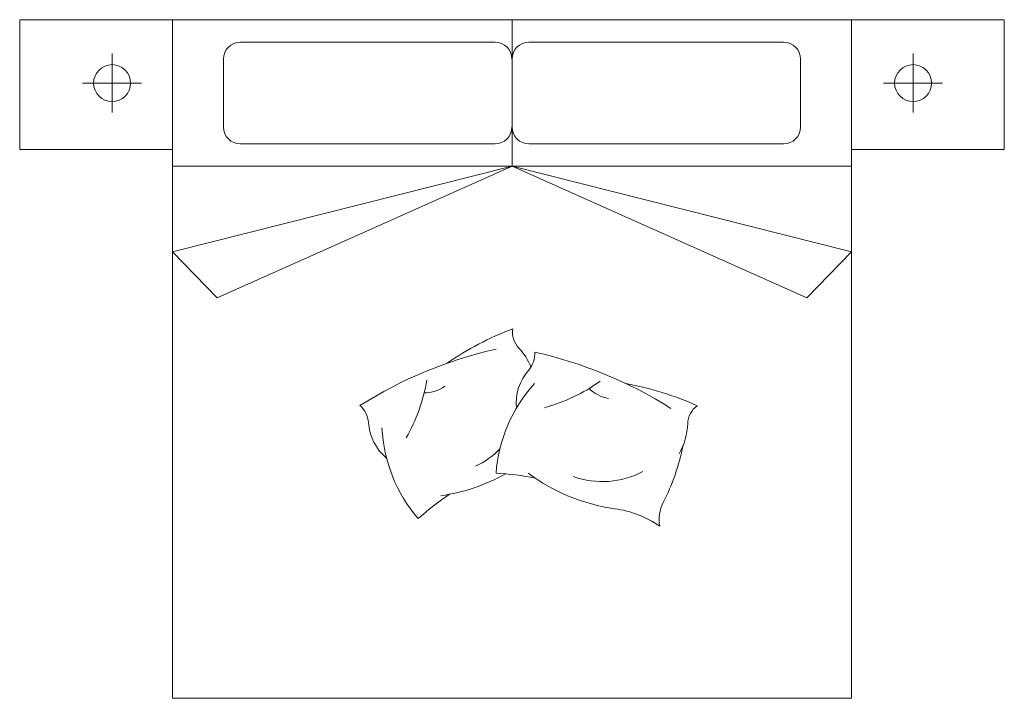
# Model space of a CAD drawing. Units: inches. Extents: x 1994 to 3075, y 3517 to 3950.
# Tile 9 of 58: x 1993.9962 to 1994.1, y 3553.8118 to 3553.8833. Entities that reach past the tile are written whole.
import ezdxf

# ---------------------------------------------------------------- set-up
doc = ezdxf.new("R2010")
doc.units = ezdxf.units.IN
doc.layers.add('A-FURN-REFR', color=8, linetype='Continuous', lineweight=13)

msp = doc.modelspace()

# ---------------------------------------------------------------- linework, layer by layer
at = {"layer": 'A-FURN-REFR'}
for p, q in [((1994.012329846586, 3553.883333005121), (1993.996223905283, 3553.883333005121)), ((1993.996223905283, 3553.883333005121), (1993.996223905283, 3553.869645257469)), ((1994.012329846586, 3553.869645257469), (1994.012329846586, 3553.883333005121)), ((1994.012329846586, 3553.883333005121), (1994.048120827259, 3553.883333005121)), ((1994.083911807932, 3553.883333005121), (1994.048120827259, 3553.883333005121)), ((1994.048120827259, 3553.883333005121), (1994.048120827259, 3553.867882559587)), ((1994.083911807932, 3553.869645257469), (1994.083911807932, 3553.883333005121)), ((1994.083911807932, 3553.883333005121), (1994.100017749235, 3553.883333005121)), ((1994.100017749235, 3553.883333005121), (1994.100017749235, 3553.869645257469)), ((1994.01948804272, 3553.880961535712), (1994.046331278225, 3553.880961535712)), ((1994.049910376293, 3553.880961535712), (1994.076753611797, 3553.880961535712)), ((1994.005960738941, 3553.873533480461), (1994.005960738941, 3553.879759345534)), ((1994.090399034003, 3553.873533480461), (1994.090399034003, 3553.879759345534)), ((1994.017698493687, 3553.872013790544), (1994.017698493687, 3553.879171986678)), ((1994.048120827259, 3553.872013790544), (1994.048120827259, 3553.879171986678)), ((1994.078543160831, 3553.879171986678), (1994.078543160831, 3553.872013790544)), ((1994.002847806404, 3553.876646412997), (1994.009073671477, 3553.876646412997)), ((1994.093511966539, 3553.876646412997), (1994.087286101467, 3553.876646412997)), ((1994.01948804272, 3553.87022424151), (1994.046331278225, 3553.87022424151)), ((1994.049910376293, 3553.87022424151), (1994.076753611797, 3553.87022424151)), ((1993.996223905283, 3553.869645257469), (1994.012329846586, 3553.869645257469)), ((1994.012329846586, 3553.811751043775), (1994.012329846586, 3553.869645257469)), ((1994.083911807932, 3553.811751043775), (1994.083911807932, 3553.869645257469)), ((1994.100017749235, 3553.869645257469), (1994.083911807932, 3553.869645257469)), ((1994.048120827259, 3553.867882559587), (1994.012320226156, 3553.858847132768)), ((1994.012329846586, 3553.867882559587), (1994.048120827259, 3553.867882559587)), ((1994.017045201164, 3553.854006547214), (1994.048120827259, 3553.867882559587)), ((1994.083911807932, 3553.867882559587), (1994.048120827259, 3553.867882559587)), ((1994.079196453354, 3553.854006547214), (1994.048120827259, 3553.867882559587)), ((1994.048120827259, 3553.867882559587), (1994.083921428361, 3553.858847132768)), ((1994.012320226156, 3553.858847132768), (1994.017045201164, 3553.854006547214)), ((1994.083921428361, 3553.858847132768), (1994.079196453354, 3553.854006547214)), ((1994.048120827259, 3553.811751043775), (1994.012329846586, 3553.811751043775)), ((1994.048120827259, 3553.811751043775), (1994.083911807932, 3553.811751043775))]:
    msp.add_line(p, q, dxfattribs=at)
for centre in [(1994.005960738941, 3553.876646412997), (1994.090399034003, 3553.876646412997)]:
    msp.add_circle(centre, 0.0019455828353276, dxfattribs=at)
for centre, radius, start, end in [((1994.01948804272, 3553.879171986678), 0.0017895490336435, 90, 180), ((1994.046331278225, 3553.879171986678), 0.0017895490336435, 0, 90), ((1994.049910376293, 3553.879171986678), 0.0017895490336435, 90, 180), ((1994.076753611797, 3553.879171986678), 0.0017895490336435, 0, 90), ((1994.01948804272, 3553.872013790544), 0.0017895490336435, 180, 270), ((1994.046331278225, 3553.872013790544), 0.0017895490336435, 270, 0), ((1994.049910376293, 3553.872013790544), 0.0017895490336435, 180, 270), ((1994.076753611797, 3553.872013790544), 0.0017895490336435, 270, 0), ((1994.060019502018, 3553.819733721454), 0.0331744460675131, 110.8823159298724, 124.5017030449515), ((1994.05065701652, 3553.850388247477), 0.0024860101449681, 172.1197168712306, 222.9397178838013), ((1994.056330439837, 3553.804465185678), 0.0452051219196895, 102.6334274117044, 122.4229229559715), ((1994.043802612966, 3553.844009882362), 0.0068770229974093, 23.06813348750885, 42.93971788380129), ((1994.04795839511, 3553.848064786977), 0.0025622673191785, 318.5500264992555, 4.47467281546091), ((1994.040685746642, 3553.804140649479), 0.0452051219196895, 57.654769534688, 77.44426507900442), ((1994.0538223304, 3553.842885935786), 0.0052611741707113, 138.5500264992554, 185.6431234876255), ((1994.030197958302, 3553.833545876559), 0.0238846517600035, 33.43324039147294, 33.44627937316185), ((1994.020889474917, 3553.848368145685), 0.0185020874209313, 330.3454935344927, 350.5126648384766), ((1994.046648381905, 3553.860247501756), 0.0185020874209313, 285.3668356574626, 305.534006961408), ((1994.0388715195, 3553.847714899879), 0.0037447944261748, 269.8428349959402, 305.6126069524626), ((1994.062273700727, 3553.834308027239), 0.0158815977655281, 137.8802473178581, 175.7484831308576), ((1994.058906600537, 3553.847074926706), 0.0037447944261748, 224.8641771190216, 260.6339490755313), ((1994.054087741859, 3553.812333566462), 0.0331744460675131, 65.90365805271031, 79.52304516794653), ((1994.030427409944, 3553.840676431349), 0.0025622673191785, 3.528684376760561, 49.45333069284981), ((1994.045927454043, 3553.842105836766), 0.0026721496709441, 5.54816698551457, 5.64312348762549), ((1994.069132946959, 3553.840635472827), 0.0024860101449681, 127.1410589942614, 177.9610600071594), ((1994.038236019051, 3553.841157950364), 0.0052611741707113, 183.5286843767605, 230.6217813648581), ((1994.050277503457, 3553.841063988989), 0.0158815977655281, 182.8589051950864, 220.7271410079812), ((1994.059775841764, 3553.840968597427), 0.0068770229974093, 330.0742520930186, 357.9610600071594), ((1994.040318100982, 3553.844497526634), 0.0091653644451756, 295.570427315862, 315.3772891878563), ((1994.042755902698, 3553.843183031926), 0.0238846517600035, 333.1334166378931, 348.4676214958053), ((1994.033202827192, 3553.835025690839), 0.0026721496709441, 50.52682486300737, 50.62178136485808), ((1994.037841907216, 3553.852633649893), 0.0197112589485322, 278.0968847510169, 299.1559945633841), ((1994.045193933864, 3553.808556233169), 0.0269577946075271, 78.44814032526723, 87.35960599722004), ((1994.061655069266, 3553.851282078094), 0.0197112589485322, 233.1182268740081, 262.1548841372723), ((1994.057655690201, 3553.843776546511), 0.0091653644451756, 250.591769438949, 297.77212499891), ((1994.056398270853, 3553.810775219775), 0.0269577946075271, 123.4267982025162, 132.338263874535), ((1994.057483410291, 3553.821005548611), 0.0108513158151594, 55.1220542741174, 82.15488413760009), ((1994.067627928503, 3553.830582967402), 0.0039968706823008, 153.1334166378931, 189.7272312675173)]:
    msp.add_arc(centre, radius, start, end, dxfattribs=at)

doc.saveas('drawing.dxf')
